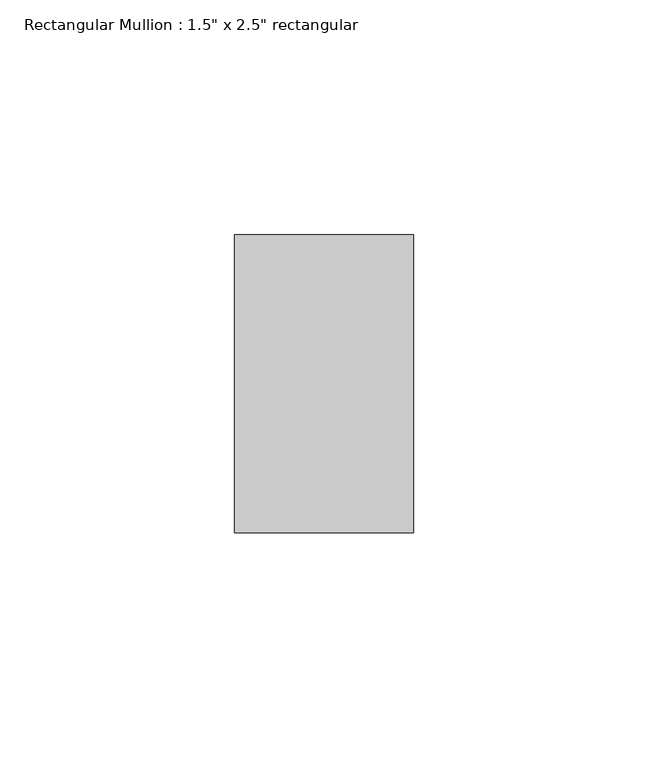
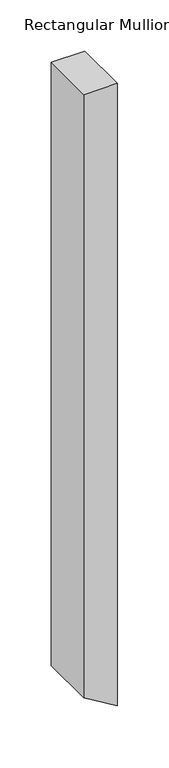
"""IFC4 building model written with IfcOpenShell, lengths in millimetres: member geometry."""

from ifc_helpers import new_model, si_unit, frame, origin, place, context, project, spatial, polyline, outline, extrude, source, transform, mapped, element, save


def member_99ded25b(model_context):
    return source(origin(), model_context, "Body", "SweptSolid", [
        extrude(outline(polyline([(0.0, 19.05), (0.0, -19.05), (-719.3609514, -19.05), (-742.0054653, 19.05), (0.0, 19.05)])), frame((0.0, -31.75, 0.0), z_axis=(0.0, 1.0, 0.0), x_axis=(0.0, 0.0, 1.0)), (0.0, 0.0, 1.0), 63.5),
    ])


if __name__ == "__main__":
    model = new_model("IFC4")
    model_context = context("Model", 3, world=origin())
    ifc_project = project(units=[si_unit("LENGTHUNIT", "METRE", prefix="MILLI")], contexts=[model_context])
    site = spatial("IfcSite", under=ifc_project)
    building = spatial("IfcBuilding", under=site)
    placement = place(None, origin())
    member_shape = member_99ded25b(model_context)
    element("IfcMember", 1, ObjectType="Rectangular Mullion : 1.5\" x 2.5\" rectangular", at=placement, inside=building, context=model_context, shape_type="MappedRepresentation", body=[
        mapped(member_shape, transform((0.0, 0.0, 0.0), x_axis=(1.0, 0.0, 0.0), y_axis=(0.0, 1.0, 0.0), z_axis=(0.0, 0.0, 1.0))),
    ])
    save(model, "model.ifc")

# Revit data of these elements
# Type "Rectangular Mullion : 1.5\" x 2.5\" rectangular"
#   built-in parameter 1007304 = 0.208333 (stored number, unit not read)
#   built-in parameter 1007301 = 0.0625 (stored number, unit not read)
#   built-in parameter 1007300 = 0.0625 (stored number, unit not read)
